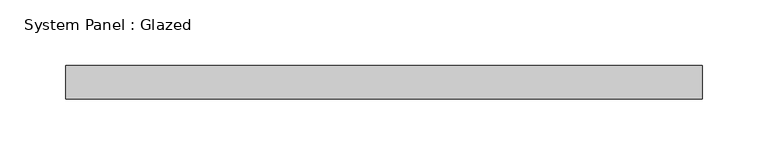
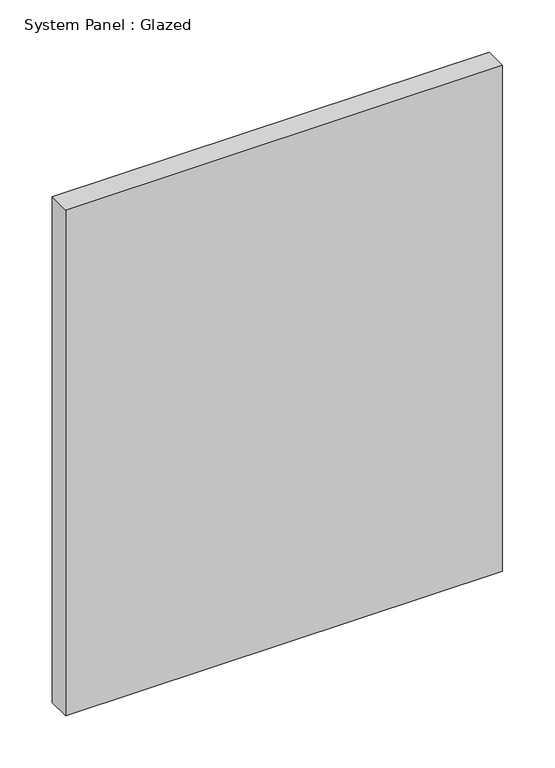
"""IFC4 building model written with IfcOpenShell, lengths in millimetres: plate geometry, System Panel : Glazed."""

from ifc_helpers import new_model, si_unit, origin, origin_with_axes, place, context, project, spatial, polyline, outline, extrude, source, transform, mapped, element, save


def system_panel_glazed_2bcfbbac(model_context):
    return source(origin(), model_context, "Body", "SweptSolid", [
        extrude(outline(polyline([(241.3, 19.05), (-241.3, 19.05), (-241.3, 44.45), (241.3, 44.45), (241.3, 19.05)])), origin_with_axes(), (0.0, 0.0, 1.0), 590.55),
    ])


if __name__ == "__main__":
    model = new_model("IFC4")
    model_context = context("Model", 3, world=origin())
    ifc_project = project(units=[si_unit("LENGTHUNIT", "METRE", prefix="MILLI")], contexts=[model_context])
    site = spatial("IfcSite", under=ifc_project)
    building = spatial("IfcBuilding", under=site)
    placement = place(None, origin())
    system_panel_glazed_shape = system_panel_glazed_2bcfbbac(model_context)
    element("IfcPlate", 1, ObjectType="System Panel : Glazed", at=placement, inside=building, context=model_context, shape_type="MappedRepresentation", body=[
        mapped(system_panel_glazed_shape, transform((0.0, 0.0, 0.0), x_axis=(1.0, 0.0, 0.0), y_axis=(0.0, 1.0, 0.0), z_axis=(0.0, 0.0, 1.0))),
    ])
    save(model, "model.ifc")

# Revit data of these elements
# Type "System Panel : Glazed"
#   Construction Type Id = "GSP4R"
#   Analytic Construction = "1/8 in Pilkington single glazing"
#   Visual Light Transmittance = 0.9
#   Solar Heat Gain Coefficient = 0.86
#   Heat Transfer Coefficient (U) = 1.18115 BTU/(h·ft²·°F)
#   Define Thermal Properties by = 1
# Element 1 (IfcPlate, "System Panel : Glazed")
#   Materials on its faces: "Glass"
# Materials
#   "Glass": class "Glass", colour RGB 0 128 192, transparency 0.75, Description = "Soda Lime Glass", Cost = 0
